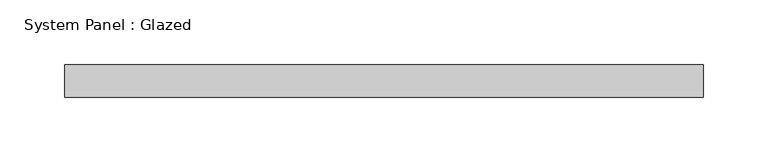
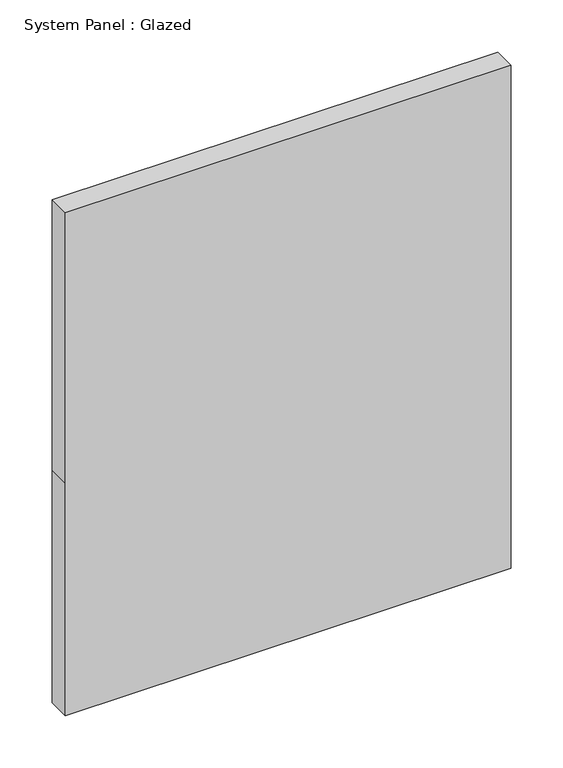
"""IFC4 building model written with IfcOpenShell, lengths in millimetres: plate geometry, System Panel : Glazed."""

from ifc_helpers import new_model, si_unit, frame, origin, place, context, project, spatial, polyline, outline, extrude, source, transform, mapped, element, save


def system_panel_glazed_d8783796(model_context):
    return source(origin(), model_context, "Body", "SweptSolid", [
        extrude(outline(polyline([(0.0, -247.65), (0.0, 247.65), (273.05, 247.65), (590.55, 247.65), (590.55, -247.65), (273.05, -247.65), (0.0, -247.65)])), frame((0.0, 19.05, 0.0), z_axis=(0.0, 1.0, 0.0), x_axis=(0.0, 0.0, 1.0)), (0.0, 0.0, 1.0), 25.4),
    ])


if __name__ == "__main__":
    model = new_model("IFC4")
    model_context = context("Model", 3, world=origin())
    ifc_project = project(units=[si_unit("LENGTHUNIT", "METRE", prefix="MILLI")], contexts=[model_context])
    site = spatial("IfcSite", under=ifc_project)
    building = spatial("IfcBuilding", under=site)
    placement = place(None, origin())
    system_panel_glazed_shape = system_panel_glazed_d8783796(model_context)
    element("IfcPlate", 1, ObjectType="System Panel : Glazed", at=placement, inside=building, context=model_context, shape_type="MappedRepresentation", body=[
        mapped(system_panel_glazed_shape, transform((0.0, 0.0, 0.0), x_axis=(1.0, 0.0, 0.0), y_axis=(0.0, 1.0, 0.0), z_axis=(0.0, 0.0, 1.0))),
    ])
    save(model, "model.ifc")

# Revit data of these elements
# Type "System Panel : Glazed"
#   Construction Type Id = "GSP4R"
#   Analytic Construction = "1/8 in Pilkington single glazing"
#   Visual Light Transmittance = 0.9
#   Solar Heat Gain Coefficient = 0.86
#   Heat Transfer Coefficient (U) = 1.18115 BTU/(h·ft²·°F)
#   Define Thermal Properties by = 1
# Element 1 (IfcPlate, "System Panel : Glazed")
#   Materials on its faces: "Glass"
# Materials
#   "Glass": class "Glass", colour RGB 0 128 192, transparency 0.75, Description = "Soda Lime Glass", Cost = 0
